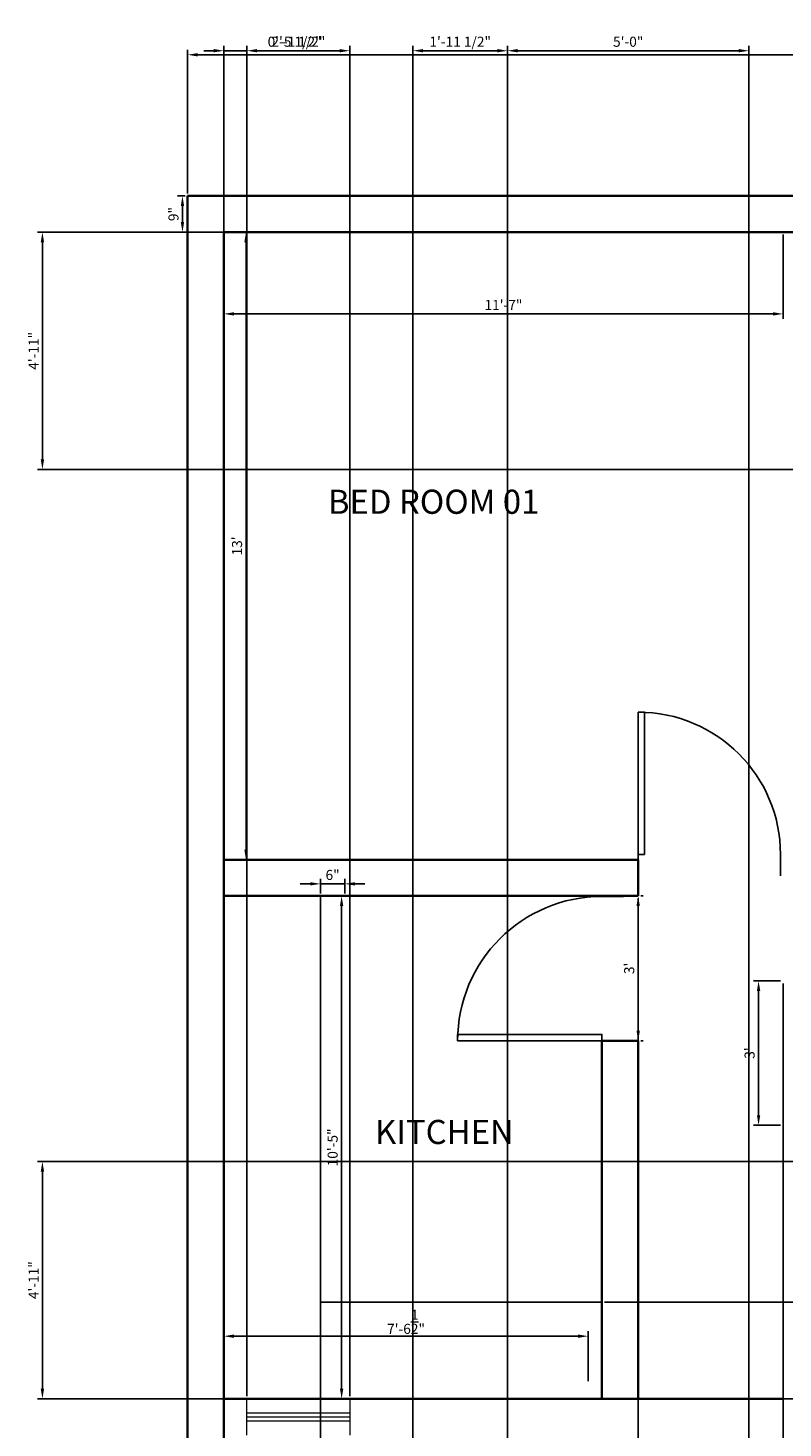
# Model space of a CAD drawing. Units: inches. Extents: x 2178 to 2667, y 1439 to 2239.
# Tile 4 of 5: x 2178 to 2366, y 1891 to 2239. Entities that reach past the tile are written whole.
import ezdxf

# ---------------------------------------------------------------- set-up
doc = ezdxf.new("R2010")
doc.units = ezdxf.units.IN
for name, color, linetype, lineweight in [('A-ANNO-DIMS', 2, 'Continuous', 18), ('A-AREA-IDEN', 7, 'Continuous', 18), ('A-DOOR', 3, 'Continuous', 25), ('A-FLOR-FIXT', 8, 'Continuous', 25), ('A-GLAZ', 4, 'Continuous', 18), ('A-WALL', 7, 'Continuous', 35)]:
    doc.layers.add(name, color=color, linetype=linetype, lineweight=lineweight)
doc.styles.get("Standard").update_dxf_attribs({"font": 'arial.ttf'})
doc.dimstyles.new('Copy of ISO-25', dxfattribs={"dimtxt": 2.5, "dimasz": 2.5, "dimexe": 1.25, "dimexo": 0.625, "dimtad": 1, "dimdec": 1, "dimlunit": 4, "dimtxsty": 'Standard', "dimcen": 2.5, "dimadec": 0, "dimazin": 0, "dimtfac": 1, "dimtdec": 1, "dimtmove": 0, "dimatfit": 3, "dimfxl": 1, "dimarcsym": 0})

# ---------------------------------------------------------------- blocks, each defined once
blk = doc.blocks.new('*D1')
at = {"layer": 'A-ANNO-DIMS', "color": 0, "lineweight": -2, "transparency": 16777216}
for p, q in [((2226.53, 2187.41), (2226.53, 2166.47)), ((2365.53, 2187.41), (2365.53, 2166.47)), ((2229.03, 2167.72), (2363.03, 2167.72))]:
    blk.add_line(p, q, dxfattribs=at)
at = {"layer": 'A-ANNO-DIMS', "color": 0, "transparency": 16777216}
for points in [[(2229.03, 2168.13), (2229.03, 2167.3), (2226.53, 2167.72)], [(2363.03, 2168.13), (2363.03, 2167.3), (2365.53, 2167.72)]]:
    blk.add_solid(points, dxfattribs=at)
at = {"layer": 'Defpoints', "color": 0, "transparency": 16777216}
for p in [(2226.53, 2188.03), (2365.53, 2188.03), (2365.53, 2167.72)]:
    blk.add_point(p, dxfattribs=at)
at = {"layer": 'A-ANNO-DIMS', "color": 0, "transparency": 16777216, "insert": (2296.03, 2169.6), "char_height": 2.5, "attachment_point": 5}
blk.add_mtext('11\'-7"', dxfattribs=at)
blk = doc.blocks.new('*D4')
at = {"layer": 'A-ANNO-DIMS', "color": 0, "lineweight": -2, "transparency": 16777216}
for p, q in [((2226.53, 1898.66), (2226.53, 1914.85)), ((2317.09, 1902.4), (2317.09, 1914.85)), ((2314.59, 1913.6), (2229.03, 1913.6))]:
    blk.add_line(p, q, dxfattribs=at)
at = {"layer": 'A-ANNO-DIMS', "color": 0, "transparency": 16777216}
for points in [[(2229.03, 1914.02), (2229.03, 1913.19), (2226.53, 1913.6)], [(2314.59, 1914.02), (2314.59, 1913.19), (2317.09, 1913.6)]]:
    blk.add_solid(points, dxfattribs=at)
at = {"layer": 'Defpoints', "color": 0, "transparency": 16777216}
for p in [(2226.53, 1913.6), (2317.09, 1901.78), (2226.53, 1898.03)]:
    blk.add_point(p, dxfattribs=at)
at = {"layer": 'A-ANNO-DIMS', "color": 0, "transparency": 16777216, "insert": (2271.81, 1917.18), "char_height": 2.5, "attachment_point": 5}
blk.add_mtext('7\'-6{\\H1x;\\S1/2;}"', dxfattribs=at)
blk = doc.blocks.new('*D5')
at = {"layer": 'A-ANNO-DIMS', "color": 0, "lineweight": -2, "transparency": 16777216}
for p, q in [((2227.15, 2023.03), (2257.05, 2023.03)), ((2255.8, 2020.53), (2255.8, 1900.53)), ((2227.15, 1898.03), (2257.05, 1898.03))]:
    blk.add_line(p, q, dxfattribs=at)
at = {"layer": 'A-ANNO-DIMS', "color": 0, "transparency": 16777216}
for points in [[(2255.39, 2020.53), (2256.22, 2020.53), (2255.8, 2023.03)], [(2255.39, 1900.53), (2256.22, 1900.53), (2255.8, 1898.03)]]:
    blk.add_solid(points, dxfattribs=at)
at = {"layer": 'Defpoints', "color": 0, "transparency": 16777216}
for p in [(2226.53, 2023.03), (2226.53, 1898.03), (2255.8, 1898.03)]:
    blk.add_point(p, dxfattribs=at)
at = {"layer": 'A-ANNO-DIMS', "color": 0, "transparency": 16777216, "insert": (2253.9, 1960.53), "char_height": 2.5, "attachment_point": 5, "rotation": 90}
blk.add_mtext('10\'-5"', dxfattribs=at)
blk = doc.blocks.new('*D10')
at = {"layer": 'A-ANNO-DIMS', "color": 0, "lineweight": -2, "transparency": 16777216}
for p, q in [((2227.15, 2188.03), (2233.29, 2188.03)), ((2232.04, 2185.53), (2232.04, 2034.53)), ((2227.15, 2032.03), (2233.29, 2032.03))]:
    blk.add_line(p, q, dxfattribs=at)
at = {"layer": 'A-ANNO-DIMS', "color": 0, "transparency": 16777216}
for points in [[(2231.62, 2185.53), (2232.45, 2185.53), (2232.04, 2188.03)], [(2231.62, 2034.53), (2232.45, 2034.53), (2232.04, 2032.03)]]:
    blk.add_solid(points, dxfattribs=at)
at = {"layer": 'Defpoints', "color": 0, "transparency": 16777216}
for p in [(2226.53, 2188.03), (2226.53, 2032.03), (2232.04, 2032.03)]:
    blk.add_point(p, dxfattribs=at)
at = {"layer": 'A-ANNO-DIMS', "color": 0, "transparency": 16777216, "insert": (2230.13, 2110.03), "char_height": 2.5, "attachment_point": 5, "rotation": 90}
blk.add_mtext("13'", dxfattribs=at)
blk = doc.blocks.new('*U24')
for p, q in [((0, 0), (0, -6)), ((40, 0), (40, -6))]:
    blk.add_line(p, q)
blk.add_lwpolyline([(0, 0), (0, 40), (1.75, 40), (1.75, 0)], close=True)
blk.add_arc((0, 0), 40, 0, 90)
blk = doc.blocks.new('*D36')
at = {"layer": 'A-ANNO-DIMS', "color": 0, "lineweight": -2, "transparency": 16777216}
for p, q in [((2330.15, 2023.03), (2330.78, 2023.03)), ((2329.53, 2020.53), (2329.53, 1989.53)), ((2330.15, 1987.03), (2330.78, 1987.03))]:
    blk.add_line(p, q, dxfattribs=at)
at = {"layer": 'A-ANNO-DIMS', "color": 0, "transparency": 16777216}
for points in [[(2329.11, 2020.53), (2329.94, 2020.53), (2329.53, 2023.03)], [(2329.11, 1989.53), (2329.94, 1989.53), (2329.53, 1987.03)]]:
    blk.add_solid(points, dxfattribs=at)
at = {"layer": 'Defpoints', "color": 0, "transparency": 16777216}
for p in [(2329.53, 2023.03), (2329.53, 1987.03), (2329.53, 1987.03)]:
    blk.add_point(p, dxfattribs=at)
at = {"layer": 'A-ANNO-DIMS', "color": 0, "transparency": 16777216, "insert": (2327.62, 2005.03), "char_height": 2.5, "attachment_point": 5, "rotation": 90}
blk.add_mtext("3'", dxfattribs=at)
blk = doc.blocks.new('*D37')
at = {"layer": 'A-ANNO-DIMS', "color": 0, "lineweight": -2, "transparency": 16777216}
for p, q in [((2364.9, 2001.92), (2358.2, 2001.92)), ((2359.45, 1999.42), (2359.45, 1968.53)), ((2364.9, 1966.03), (2358.2, 1966.03))]:
    blk.add_line(p, q, dxfattribs=at)
at = {"layer": 'A-ANNO-DIMS', "color": 0, "transparency": 16777216}
for points in [[(2359.04, 1999.42), (2359.87, 1999.42), (2359.45, 2001.92)], [(2359.04, 1968.53), (2359.87, 1968.53), (2359.45, 1966.03)]]:
    blk.add_solid(points, dxfattribs=at)
at = {"layer": 'Defpoints', "color": 0, "transparency": 16777216}
for p in [(2365.53, 2001.92), (2359.45, 1966.03), (2365.53, 1966.03)]:
    blk.add_point(p, dxfattribs=at)
at = {"layer": 'A-ANNO-DIMS', "color": 0, "transparency": 16777216, "insert": (2357.55, 1983.98), "char_height": 2.5, "attachment_point": 5, "rotation": 90}
blk.add_mtext("3'", dxfattribs=at)
blk = doc.blocks.new('*D42')
at = {"layer": 'A-ANNO-DIMS', "color": 0, "lineweight": -2, "transparency": 16777216}
for p, q in [((2217.53, 2197.66), (2217.53, 2233.38)), ((2220.03, 2232.13), (2575.03, 2232.13)), ((2577.53, 2197.66), (2577.53, 2233.38))]:
    blk.add_line(p, q, dxfattribs=at)
at = {"layer": 'A-ANNO-DIMS', "color": 0, "transparency": 16777216}
for points in [[(2220.03, 2232.54), (2220.03, 2231.71), (2217.53, 2232.13)], [(2575.03, 2232.54), (2575.03, 2231.71), (2577.53, 2232.13)]]:
    blk.add_solid(points, dxfattribs=at)
at = {"layer": 'Defpoints', "color": 0, "transparency": 16777216}
for p in [(2577.53, 2232.13), (2217.53, 2197.03), (2577.53, 2197.03)]:
    blk.add_point(p, dxfattribs=at)
at = {"layer": 'A-ANNO-DIMS', "color": 0, "transparency": 16777216, "insert": (2397.53, 2234.03), "char_height": 2.5, "attachment_point": 5}
blk.add_mtext("30'", dxfattribs=at)
blk = doc.blocks.new('*D43')
at = {"layer": 'A-ANNO-DIMS', "color": 0, "lineweight": -2, "transparency": 16777216}
for p, q in [((2216.9, 2197.03), (2214.99, 2197.03)), ((2216.24, 2194.53), (2216.24, 2190.53)), ((2216.9, 2188.03), (2214.99, 2188.03))]:
    blk.add_line(p, q, dxfattribs=at)
at = {"layer": 'A-ANNO-DIMS', "color": 0, "transparency": 16777216}
for points in [[(2215.82, 2194.53), (2216.65, 2194.53), (2216.24, 2197.03)], [(2215.82, 2190.53), (2216.65, 2190.53), (2216.24, 2188.03)]]:
    blk.add_solid(points, dxfattribs=at)
at = {"layer": 'Defpoints', "color": 0, "transparency": 16777216}
for p in [(2217.53, 2197.03), (2216.24, 2188.03), (2217.53, 2188.03)]:
    blk.add_point(p, dxfattribs=at)
at = {"layer": 'A-ANNO-DIMS', "color": 0, "transparency": 16777216, "insert": (2214.34, 2192.53), "char_height": 2.5, "attachment_point": 5, "rotation": 90}
blk.add_mtext('9"', dxfattribs=at)
blk = doc.blocks.new('*D44')
at = {"layer": 'A-ANNO-DIMS', "color": 0, "lineweight": -2, "transparency": 16777216}
for p, q in [((2248.03, 2026.04), (2245.53, 2026.04)), ((2250.53, 2023.66), (2250.53, 2027.29)), ((2250.53, 2026.04), (2256.59, 2026.04)), ((2256.59, 2023.66), (2256.59, 2027.29)), ((2259.09, 2026.04), (2261.59, 2026.04))]:
    blk.add_line(p, q, dxfattribs=at)
at = {"layer": 'A-ANNO-DIMS', "color": 0, "transparency": 16777216}
for points in [[(2248.03, 2026.46), (2248.03, 2025.63), (2250.53, 2026.04)], [(2259.09, 2026.46), (2259.09, 2025.63), (2256.59, 2026.04)]]:
    blk.add_solid(points, dxfattribs=at)
at = {"layer": 'Defpoints', "color": 0, "transparency": 16777216}
for p in [(2256.59, 2026.04), (2250.53, 2023.03), (2256.59, 2023.03)]:
    blk.add_point(p, dxfattribs=at)
at = {"layer": 'A-ANNO-DIMS', "color": 0, "transparency": 16777216, "insert": (2253.56, 2027.94), "char_height": 2.5, "attachment_point": 5}
blk.add_mtext('6"', dxfattribs=at)
blk = doc.blocks.new('*D48')
at = {"layer": 'A-ANNO-DIMS', "color": 0, "lineweight": -2, "transparency": 16777216}
for p, q in [((2437.9, 2188.03), (2180.18, 2188.03)), ((2181.43, 2185.53), (2181.43, 2131.53)), ((2437.9, 2129.03), (2180.18, 2129.03))]:
    blk.add_line(p, q, dxfattribs=at)
at = {"layer": 'A-ANNO-DIMS', "color": 0, "transparency": 16777216}
for points in [[(2181.01, 2185.53), (2181.84, 2185.53), (2181.43, 2188.03)], [(2181.01, 2131.53), (2181.84, 2131.53), (2181.43, 2129.03)]]:
    blk.add_solid(points, dxfattribs=at)
at = {"layer": 'Defpoints', "color": 0, "transparency": 16777216}
for p in [(2438.53, 2188.03), (2181.43, 2129.03), (2438.53, 2129.03)]:
    blk.add_point(p, dxfattribs=at)
at = {"layer": 'A-ANNO-DIMS', "color": 0, "transparency": 16777216, "insert": (2179.55, 2158.53), "char_height": 2.5, "attachment_point": 5, "rotation": 90}
blk.add_mtext('4\'-11"', dxfattribs=at)
blk = doc.blocks.new('*D49')
at = {"layer": 'A-ANNO-DIMS', "color": 0, "lineweight": -2, "transparency": 16777216}
for p, q in [((2567.9, 1957.03), (2180.18, 1957.03)), ((2181.43, 1954.53), (2181.43, 1900.53)), ((2567.9, 1898.03), (2180.18, 1898.03))]:
    blk.add_line(p, q, dxfattribs=at)
at = {"layer": 'A-ANNO-DIMS', "color": 0, "transparency": 16777216}
for points in [[(2181.01, 1954.53), (2181.84, 1954.53), (2181.43, 1957.03)], [(2181.01, 1900.53), (2181.84, 1900.53), (2181.43, 1898.03)]]:
    blk.add_solid(points, dxfattribs=at)
at = {"layer": 'Defpoints', "color": 0, "transparency": 16777216}
for p in [(2568.53, 1957.03), (2181.43, 1898.03), (2568.53, 1898.03)]:
    blk.add_point(p, dxfattribs=at)
at = {"layer": 'A-ANNO-DIMS', "color": 0, "transparency": 16777216, "insert": (2179.55, 1927.53), "char_height": 2.5, "attachment_point": 5, "rotation": 90}
blk.add_mtext('4\'-11"', dxfattribs=at)
blk = doc.blocks.new('*D51')
at = {"layer": 'A-ANNO-DIMS', "color": 0, "lineweight": -2, "transparency": 16777216}
for p, q in [((2273.53, 1597.16), (2273.53, 2234.38)), ((2297.04, 1597.16), (2297.04, 2234.38)), ((2276.03, 2233.13), (2294.54, 2233.13))]:
    blk.add_line(p, q, dxfattribs=at)
at = {"layer": 'A-ANNO-DIMS', "color": 0, "transparency": 16777216}
for points in [[(2276.03, 2233.55), (2276.03, 2232.72), (2273.53, 2233.13)], [(2294.54, 2233.55), (2294.54, 2232.72), (2297.04, 2233.13)]]:
    blk.add_solid(points, dxfattribs=at)
at = {"layer": 'Defpoints', "color": 0, "transparency": 16777216}
for p in [(2297.04, 2233.13), (2273.53, 1596.53), (2297.04, 1596.53)]:
    blk.add_point(p, dxfattribs=at)
at = {"layer": 'A-ANNO-DIMS', "color": 0, "transparency": 16777216, "insert": (2285.28, 2235.05), "char_height": 2.5, "attachment_point": 5}
blk.add_mtext('1\'-11 1/2"', dxfattribs=at)
blk = doc.blocks.new('*D52')
at = {"layer": 'A-ANNO-DIMS', "color": 0, "lineweight": -2, "transparency": 16777216}
for p, q in [((2297.04, 1597.16), (2297.04, 2234.38)), ((2357.04, 1597.16), (2357.04, 2234.38)), ((2299.54, 2233.13), (2354.54, 2233.13))]:
    blk.add_line(p, q, dxfattribs=at)
at = {"layer": 'A-ANNO-DIMS', "color": 0, "transparency": 16777216}
for points in [[(2299.54, 2233.55), (2299.54, 2232.72), (2297.04, 2233.13)], [(2354.54, 2233.55), (2354.54, 2232.72), (2357.04, 2233.13)]]:
    blk.add_solid(points, dxfattribs=at)
at = {"layer": 'Defpoints', "color": 0, "transparency": 16777216}
for p in [(2357.04, 2233.13), (2297.04, 1596.53), (2357.04, 1596.53)]:
    blk.add_point(p, dxfattribs=at)
at = {"layer": 'A-ANNO-DIMS', "color": 0, "transparency": 16777216, "insert": (2327.04, 2235.04), "char_height": 2.5, "attachment_point": 5}
blk.add_mtext('5\'-0"', dxfattribs=at)
blk = doc.blocks.new('*D61')
at = {"layer": 'A-ANNO-DIMS', "color": 0, "lineweight": -2, "transparency": 16777216}
for p, q in [((2232.26, 1898.66), (2232.26, 2234.38)), ((2257.84, 1898.66), (2257.84, 2234.38)), ((2234.76, 2233.13), (2255.34, 2233.13))]:
    blk.add_line(p, q, dxfattribs=at)
at = {"layer": 'A-ANNO-DIMS', "color": 0, "transparency": 16777216}
for points in [[(2234.76, 2233.55), (2234.76, 2232.72), (2232.26, 2233.13)], [(2255.34, 2233.55), (2255.34, 2232.72), (2257.84, 2233.13)]]:
    blk.add_solid(points, dxfattribs=at)
at = {"layer": 'Defpoints', "color": 0, "transparency": 16777216}
for p in [(2257.84, 2233.13), (2232.26, 1898.03), (2257.84, 1898.03)]:
    blk.add_point(p, dxfattribs=at)
at = {"layer": 'A-ANNO-DIMS', "color": 0, "transparency": 16777216, "insert": (2245.05, 2235.05), "char_height": 2.5, "attachment_point": 5}
blk.add_mtext('2\'-1 1/2"', dxfattribs=at)
blk = doc.blocks.new('*D62')
at = {"layer": 'A-ANNO-DIMS', "color": 0, "lineweight": -2, "transparency": 16777216}
for p, q in [((2226.53, 1898.66), (2226.53, 2234.38)), ((2232.26, 1898.66), (2232.26, 2234.38)), ((2224.03, 2233.13), (2221.53, 2233.13)), ((2226.53, 2233.13), (2232.26, 2233.13)), ((2234.76, 2233.13), (2250.98, 2233.13))]:
    blk.add_line(p, q, dxfattribs=at)
at = {"layer": 'A-ANNO-DIMS', "color": 0, "transparency": 16777216}
for points in [[(2224.03, 2233.55), (2224.03, 2232.72), (2226.53, 2233.13)], [(2234.76, 2233.55), (2234.76, 2232.72), (2232.26, 2233.13)]]:
    blk.add_solid(points, dxfattribs=at)
at = {"layer": 'Defpoints', "color": 0, "transparency": 16777216}
for p in [(2232.26, 2233.13), (2226.53, 1898.03), (2232.26, 1898.03)]:
    blk.add_point(p, dxfattribs=at)
at = {"layer": 'A-ANNO-DIMS', "color": 0, "transparency": 16777216, "insert": (2244.12, 2235.05), "char_height": 2.5, "attachment_point": 5}
blk.add_mtext('0\'-5 1/2"', dxfattribs=at)
blk = doc.blocks.new('*D67')
at = {"layer": 'A-ANNO-DIMS', "color": 0, "lineweight": -2, "transparency": 16777216}
for p, q in [((2226.53, 2022.41), (2226.53, 1439.68)), ((2250.53, 2022.41), (2250.53, 1439.68)), ((2229.03, 1440.93), (2248.03, 1440.93))]:
    blk.add_line(p, q, dxfattribs=at)
at = {"layer": 'A-ANNO-DIMS', "color": 0, "transparency": 16777216}
for points in [[(2229.03, 1441.35), (2229.03, 1440.52), (2226.53, 1440.93)], [(2248.03, 1441.35), (2248.03, 1440.52), (2250.53, 1440.93)]]:
    blk.add_solid(points, dxfattribs=at)
at = {"layer": 'Defpoints', "color": 0, "transparency": 16777216}
for p in [(2226.53, 2023.03), (2250.53, 2023.03), (2250.53, 1440.93)]:
    blk.add_point(p, dxfattribs=at)
at = {"layer": 'A-ANNO-DIMS', "color": 0, "transparency": 16777216, "insert": (2238.53, 1442.84), "char_height": 2.5, "attachment_point": 5}
blk.add_mtext('2\'-0"', dxfattribs=at)
blk = doc.blocks.new('*D68')
at = {"layer": 'A-ANNO-DIMS', "color": 0, "lineweight": -2, "transparency": 16777216}
for p, q in [((2321.15, 1922.03), (2614.88, 1922.03)), ((2613.63, 1900.53), (2613.63, 1919.53)), ((2321.15, 1898.03), (2614.88, 1898.03))]:
    blk.add_line(p, q, dxfattribs=at)
at = {"layer": 'A-ANNO-DIMS', "color": 0, "transparency": 16777216}
for points in [[(2613.21, 1919.53), (2614.04, 1919.53), (2613.63, 1922.03)], [(2613.21, 1900.53), (2614.04, 1900.53), (2613.63, 1898.03)]]:
    blk.add_solid(points, dxfattribs=at)
at = {"layer": 'Defpoints', "color": 0, "transparency": 16777216}
for p in [(2320.53, 1922.03), (2613.63, 1922.03), (2320.53, 1898.03)]:
    blk.add_point(p, dxfattribs=at)
at = {"layer": 'A-ANNO-DIMS', "color": 0, "transparency": 16777216, "insert": (2611.72, 1910.03), "char_height": 2.5, "attachment_point": 5, "rotation": 90}
blk.add_mtext('2\'-0"', dxfattribs=at)
blk = doc.blocks.new('*D69')
at = {"layer": 'A-ANNO-DIMS', "color": 0, "lineweight": -2, "transparency": 16777216}
for p, q in [((2329.53, 2022.41), (2329.53, 1439.68)), ((2365.53, 2001.3), (2365.53, 1439.68)), ((2332.03, 1440.93), (2363.03, 1440.93))]:
    blk.add_line(p, q, dxfattribs=at)
at = {"layer": 'A-ANNO-DIMS', "color": 0, "transparency": 16777216}
for points in [[(2332.03, 1441.35), (2332.03, 1440.52), (2329.53, 1440.93)], [(2363.03, 1441.35), (2363.03, 1440.52), (2365.53, 1440.93)]]:
    blk.add_solid(points, dxfattribs=at)
at = {"layer": 'Defpoints', "color": 0, "transparency": 16777216}
for p in [(2329.53, 2023.03), (2365.53, 2001.92), (2365.53, 1440.93)]:
    blk.add_point(p, dxfattribs=at)
at = {"layer": 'A-ANNO-DIMS', "color": 0, "transparency": 16777216, "insert": (2347.53, 1442.84), "char_height": 2.5, "attachment_point": 5}
blk.add_mtext('3\'-0"', dxfattribs=at)

msp = doc.modelspace()

# ---------------------------------------------------------------- linework, layer by layer
at = {"layer": 'A-FLOR-FIXT'}
for p, q in [((2226.53, 2023.03), (2250.53, 2023.03)), ((2250.53, 2023.03), (2250.53, 1898.03)), ((2250.53, 1898.03), (2250.53, 1922.03)), ((2250.53, 1922.03), (2320.53, 1922.03))]:
    msp.add_line(p, q, dxfattribs=at)
at = {"layer": 'A-GLAZ'}
for p, q in [((2232.26, 1889.03), (2232.26, 1898.03)), ((2232.26, 1898.03), (2257.84, 1898.03)), ((2257.84, 1898.03), (2257.84, 1889.03)), ((2232.26, 1894.53), (2257.84, 1894.53)), ((2232.26, 1893.53), (2257.84, 1893.53)), ((2232.26, 1892.53), (2257.84, 1892.53))]:
    msp.add_line(p, q, dxfattribs=at)
at = {"layer": 'A-WALL'}
for p, q in [((2217.53, 2197.03), (2577.53, 2197.03)), ((2217.53, 1477.03), (2217.53, 2197.03)), ((2226.53, 2188.03), (2568.53, 2188.03)), ((2226.53, 2188.03), (2365.53, 2188.03)), ((2226.53, 1805.03), (2226.53, 2188.03)), ((2329.53, 2032.03), (2226.53, 2032.03)), ((2226.53, 2032.03), (2226.53, 2023.03)), ((2329.53, 2023.03), (2329.53, 2032.03)), ((2226.53, 2023.03), (2320.53, 2023.03)), ((2226.53, 2023.03), (2226.53, 1898.03)), ((2320.53, 2023.03), (2329.53, 2023.03)), ((2329.53, 2023.03), (2329.53, 2023.03)), ((2320.53, 1898.03), (2320.53, 1987.03)), ((2320.53, 1987.03), (2329.53, 1987.03)), ((2329.53, 1987.03), (2329.53, 1898.03)), ((2226.53, 1898.03), (2365.53, 1898.03)), ((2329.53, 1898.03), (2320.53, 1898.03))]:
    msp.add_line(p, q, dxfattribs=at)

# ---------------------------------------------------------------- block references
at = {"layer": 'A-DOOR', "xscale": 0.8844272464074808, "yscale": 0.8844272464074808, "zscale": 0.8844272464074808}
msp.add_blockref('*U24', (2329.53, 2033.34), dxfattribs=at)
at = {"layer": 'A-DOOR', "xscale": 0.8971499256419678, "yscale": 0.8971499256419678, "zscale": 0.8971499256419678, "rotation": 90}
msp.add_blockref('*U24', (2320.53, 1987.03), dxfattribs=at)

# ---------------------------------------------------------------- texts
at = {"layer": 'A-AREA-IDEN'}
for s, p in [('BED ROOM 01', (2252.38, 2118.02)), ('KITCHEN', (2264.1, 1961.37))]:
    msp.add_text(s, height=6, dxfattribs=at).set_placement(p)

# ---------------------------------------------------------------- dimensions: what is measured, and where the dimension line sits
at = {"layer": 'A-ANNO-DIMS'}
for base, p1, p2, override, picture, middle in [((2232.26, 2233.13), (2226.53, 1898.03), (2232.26, 1898.03), {"dimdec": 1, "dimlfac": 1, "dimrnd": 0, "dimzin": 1, "dimdsep": 46, "dimlunit": 4, "dimfrac": 2}, '*D62', (2244.12, 2235.05)), ((2257.84, 2233.13), (2232.26, 1898.03), (2257.84, 1898.03), {"dimdec": 1, "dimlfac": 1, "dimrnd": 0, "dimzin": 1, "dimdsep": 46, "dimlunit": 4, "dimfrac": 2}, '*D61', (2245.05, 2235.05)), ((2297.04, 2233.13), (2273.53, 1596.53), (2297.04, 1596.53), {"dimdec": 1, "dimlfac": 1, "dimrnd": 0, "dimzin": 1, "dimdsep": 46, "dimlunit": 4, "dimfrac": 2}, '*D51', (2285.28, 2235.05)), ((2577.53, 2232.13), (2217.53, 2197.03), (2577.53, 2197.03), {"dimclrd": 0, "dimclre": 0, "dimclrt": 0}, '*D42', (2397.53, 2234.03)), ((2357.04, 2233.13), (2297.04, 1596.53), (2357.04, 1596.53), {"dimdec": 1, "dimlfac": 1, "dimrnd": 0, "dimzin": 1, "dimdsep": 46, "dimlunit": 4, "dimfrac": 2}, '*D52', (2327.04, 2235.04)), ((2365.53, 2167.72), (2226.53, 2188.03), (2365.53, 2188.03), {"dimclrd": 0, "dimclre": 0, "dimclrt": 0}, '*D1', (2296.03, 2169.6)), ((2256.59, 2026.04), (2250.53, 2023.03), (2256.59, 2023.03), {"dimclrd": 0, "dimclre": 0, "dimclrt": 0}, '*D44', (2253.56, 2027.94)), ((2250.53, 1440.93), (2226.53, 2023.03), (2250.53, 2023.03), {"dimdec": 1, "dimlfac": 1, "dimrnd": 0, "dimzin": 1, "dimdsep": 46, "dimlunit": 4, "dimfrac": 2}, '*D67', (2238.53, 1442.84)), ((2365.53, 1440.93), (2329.53, 2023.03), (2365.53, 2001.92), {"dimdec": 1, "dimlfac": 1, "dimrnd": 0, "dimzin": 1, "dimdsep": 46, "dimlunit": 4, "dimfrac": 2}, '*D69', (2347.53, 1442.84)), ((2226.53, 1913.6), (2317.09, 1901.78), (2226.53, 1898.03), {"dimclrd": 0, "dimclre": 0, "dimclrt": 0}, '*D4', (2271.81, 1917.18))]:
    dim = msp.add_linear_dim(base=base, p1=p1, p2=p2, dimstyle='Copy of ISO-25', override=override, dxfattribs=at)
    dim.commit()
    dim.dimension.update_dxf_attribs({"geometry": picture, "text_midpoint": middle})
for base, p1, p2, override, picture, middle in [((2216.24, 2188.03), (2217.53, 2197.03), (2217.53, 2188.03), {"dimclrd": 0, "dimclre": 0, "dimclrt": 0}, '*D43', (2214.34, 2192.53)), ((2181.43, 2129.03), (2438.53, 2188.03), (2438.53, 2129.03), {"dimdec": 1, "dimlfac": 1, "dimrnd": 0, "dimzin": 1, "dimdsep": 46, "dimlunit": 4, "dimfrac": 2}, '*D48', (2179.55, 2158.53)), ((2232.04, 2032.03), (2226.53, 2188.03), (2226.53, 2032.03), {"dimclrd": 0, "dimclre": 0, "dimclrt": 0}, '*D10', (2230.13, 2110.03)), ((2255.8, 1898.03), (2226.53, 2023.03), (2226.53, 1898.03), {"dimclrd": 0, "dimclre": 0, "dimclrt": 0}, '*D5', (2253.9, 1960.53)), ((2329.53, 1987.03), (2329.53, 2023.03), (2329.53, 1987.03), {"dimclrd": 0, "dimclre": 0, "dimclrt": 0}, '*D36', (2327.62, 2005.03)), ((2359.45, 1966.03), (2365.53, 2001.92), (2365.53, 1966.03), {"dimclrd": 0, "dimclre": 0, "dimclrt": 0}, '*D37', (2357.55, 1983.98)), ((2181.43, 1898.03), (2568.53, 1957.03), (2568.53, 1898.03), {"dimdec": 1, "dimlfac": 1, "dimrnd": 0, "dimzin": 1, "dimdsep": 46, "dimlunit": 4, "dimfrac": 2}, '*D49', (2179.55, 1927.53)), ((2613.63, 1922.03), (2320.53, 1898.03), (2320.53, 1922.03), {"dimdec": 1, "dimlfac": 1, "dimrnd": 0, "dimzin": 1, "dimdsep": 46, "dimlunit": 4, "dimfrac": 2}, '*D68', (2611.72, 1910.03))]:
    dim = msp.add_linear_dim(base=base, p1=p1, p2=p2, angle=90, dimstyle='Copy of ISO-25', override=override, dxfattribs=at)
    dim.commit()
    dim.dimension.update_dxf_attribs({"geometry": picture, "text_midpoint": middle})

doc.saveas('drawing.dxf')
